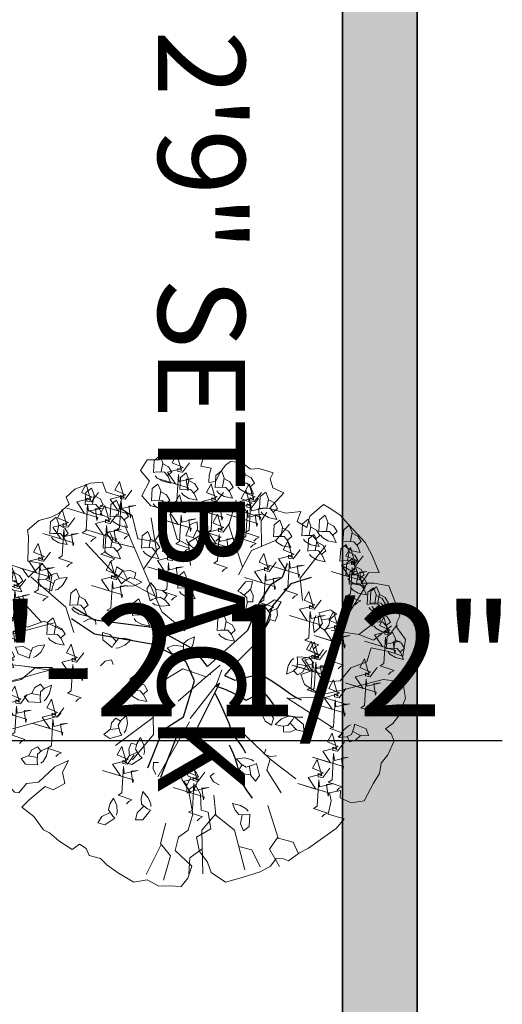
# Model space of a CAD drawing. Units: inches. Extents: x 2337 to 3570, y 1258 to 1938.
# Tile 12 of 30: x 2874 to 2913, y 1598 to 1677. Entities that reach past the tile are written whole.
import ezdxf

# ---------------------------------------------------------------- set-up
doc = ezdxf.new("R2010")
doc.units = ezdxf.units.IN
for name, color, linetype, lineweight in [('A-ANNO-DIMS', 2, 'Continuous', 18), ('A-ANNO-TEXT', 7, 'Continuous', 18), ('ARBOL', 74, 'Continuous', 13), ('C-PROP', 7, 'Continuous', 35)]:
    doc.layers.add(name, color=color, linetype=linetype, lineweight=lineweight)
doc.layers.add('C-PROP-PATT', color=251, linetype='Continuous', lineweight=13, true_color=0x636466)
doc.layers.add('TALLO', color=36, linetype='Continuous')
doc.styles.get("Standard").update_dxf_attribs({"font": 'arial.ttf'})
doc.dimstyles.new('ISO-25', dxfattribs={"dimtxt": 9, "dimasz": 2.5, "dimexe": 1.25, "dimexo": 0.625, "dimtad": 1, "dimdec": 1, "dimlunit": 3, "dimtxsty": 'Standard', "dimcen": 2.5, "dimadec": 0, "dimazin": 0, "dimtfac": 1, "dimtdec": 1, "dimtmove": 0, "dimatfit": 3, "dimfxl": 1, "dimarcsym": 0})

# ---------------------------------------------------------------- blocks, each defined once
blk = doc.blocks.new('fresno')
at = {"layer": 'ARBOL'}
for p, q in [((2.96, 0.991), (3.575, 1.984)), ((-3.638, 1.194), (-4.164, 1.76)), ((-1.151, -0.932), (-1.99, -1.556)), ((-0.974, -3.757), (-1.31, -4.423))]:
    blk.add_line(p, q, dxfattribs=at)
blk.add_lwpolyline([(0.823, 4.745), (0.566, 4.764), (0.459, 4.687), (0.336, 4.518), (0.233, 4.322), (0.087, 4.298), (0.091, 4.464), (0.14, 4.621), (-0.09, 4.659), (-0.033, 4.863), (-0.264, 4.901), (-0.483, 4.866), (-0.686, 4.924), (-1.021, 4.801), (-1.288, 4.8), (-1.431, 4.563), (-1.234, 4.327), (-1.406, 4), (-1.205, 3.778), (-0.909, 3.705), (-0.931, 3.283), (-1.122, 2.983), (-1.491, 3.043), (-1.619, 3.562), (-1.9, 3.727), (-1.851, 3.982), (-2.197, 4.084), (-2.278, 4.31), (-2.543, 4.283), (-2.896, 4.152), (-3.091, 3.971), (-3.022, 3.817), (-3.244, 3.617), (-3.424, 3.528), (-3.697, 3.455), (-3.946, 3.236), (-3.922, 3.09), (-3.94, 2.548), (-3.617, 2.495), (-3.927, 2.19), (-4.062, 2.379), (-4.443, 2.512), (-4.546, 2.316), (-4.73, 2.062), (-4.767, 1.832), (-4.671, 1.698), (-4.486, 1.667), (-4.693, 1.559), (-4.854, 1.444), (-4.934, 1.102), (-5.037, 0.905), (-5.175, 0.644), (-5.166, 0.406), (-5.024, 0.264), (-4.781, 0.153), (-4.363, 0.249), (-4.014, 0.215), (-3.783, 0.177), (-3.46, 0.124), (-3.733, 0.051), (-4.132, -0.073), (-4.404, -0.146), (-4.639, 0.011), (-4.977, -0.028), (-5.172, -0.209), (-5.113, -0.574), (-4.921, -0.843), (-4.951, -1.027), (-5.012, -1.112), (-4.95, -1.311), (-4.83, -1.592), (-4.676, -1.807), (-4.518, -1.856), (-4.529, -2.068), (-4.417, -2.394), (-4.236, -2.59), (-4.143, -2.605), (-3.967, -2.397), (-3.703, -2.37), (-3.339, -2.027), (-3.032, -1.889), (-3.169, -2.15), (-3.115, -2.396), (-3.376, -2.542), (-3.552, -2.466), (-3.909, -2.762), (-4.077, -2.924), (-3.804, -3.135), (-3.592, -3.43), (-3.461, -3.499), (-3.253, -3.676), (-2.953, -3.867), (-2.792, -3.752), (-2.642, -3.848), (-2.572, -4.001), (-2.323, -4.066), (-2.18, -4.208), (-1.926, -4.392), (-1.58, -4.591), (-1.288, -4.545), (-1.027, -4.683), (-0.788, -4.675), (-0.531, -4.693), (-0.382, -4.505), (-0.29, -4.236), (-0.66, -3.891), (-0.588, -3.595), (-0.374, -3.441), (-0.267, -3.079), (-0.368, -2.541), (-0.208, -2.426), (-0.099, -2.633), (-0.087, -2.991), (0.071, -3.04), (0.129, -3.405), (-0.185, -3.59), (-0.119, -3.909), (0.055, -4.151), (0.136, -4.377), (0.456, -4.596), (0.828, -4.491), (1.227, -4.368), (1.461, -4.241), (1.583, -4.071), (1.748, -4.075), (1.86, -4.117), (2.101, -3.944), (2.308, -3.836), (2.925, -3.393), (3.101, -3.185), (2.74, -3.078), (2.812, -2.782), (2.769, -2.61), (3.015, -2.555), (3.012, -2.721), (3.254, -2.832), (3.546, -2.785), (3.752, -2.393), (3.882, -2.177), (3.92, -1.947), (4.069, -1.758), (4.214, -1.451), (4.144, -1.297), (4.021, -1.182), (4.182, -1.067), (4.304, -0.897), (4.464, -0.497), (4.429, -0.279), (4.406, -0.133), (3.964, -0.083), (3.074, -0.315), (2.582, -0.424), (2.217, -0.197), (2.136, 0.029), (2.462, 0.141), (2.628, -0.147), (3.012, -0.116), (3.249, 0.177), (3.602, 0.308), (3.701, 0.623), (4.089, 0.535), (4.404, 0.436), (4.464, 0.805), (4.272, 1.074), (4.267, 1.193), (4.336, 1.324), (4.243, 1.623), (4.092, 2.003), (3.769, 2.057), (3.485, 2.056), (3.642, 2.291), (3.88, 2.299), (3.71, 2.706), (3.563, 2.967), (3.201, 3.358), (3.001, 3.581), (2.766, 3.738), (2.635, 3.807), (2.332, 3.549), (2.268, 3.299), (2.052, 3.429), (2.136, 3.652), (1.798, 3.613), (1.437, 3.72), (1.755, 4.071), (1.513, 4.182), (1.451, 4.381), (1.519, 4.512), (1.204, 4.611), (1.012, 4.596)], close=True, dxfattribs=at)
for points in [[(-1.104, 4.45), (-1.063, 4.399), (-0.939, 4.325), (-0.757, 4.285), (-0.82, 4.431), (-0.903, 4.527), (-1.075, 4.533), (-1.143, 4.521), (-1.126, 4.792), (-1.002, 4.891), (-0.939, 4.738), (-0.975, 4.535)], [(-0.346, 4.735), (-0.501, 4.528), (-0.605, 4.545), (-0.605, 4.614), (-0.519, 4.563), (-0.622, 4.925), (-0.726, 4.735), (-0.484, 4.632), (-0.622, 4.58), (-0.829, 4.528), (-0.657, 4.27), (-1.053, 4.39), (-0.363, 4.183), (-0.381, 4.114), (-0.415, 4.373), (-0.26, 4.39), (-0.57, 4.321), (-0.588, 4.476), (-0.622, 3.89), (-0.708, 3.839), (-0.398, 3.735), (-0.467, 3.701), (-0.519, 3.649)], [(-0.935, 4.717), (-0.809, 4.65), (-0.736, 4.529), (-0.824, 4.459)], [(0.734, 4.203), (0.775, 4.152), (0.9, 4.078), (1.082, 4.038), (1.018, 4.185), (0.936, 4.281), (0.763, 4.287), (0.696, 4.274), (0.712, 4.546), (0.837, 4.645), (0.899, 4.491), (0.863, 4.289)], [(-0.521, 4.069), (-0.48, 4.018), (-0.356, 3.944), (-0.174, 3.904), (-0.237, 4.051), (-0.32, 4.146), (-0.492, 4.152), (-0.56, 4.14), (-0.543, 4.411), (-0.419, 4.511), (-0.356, 4.357), (-0.392, 4.154)], [(0.263, 4.114), (0.304, 4.063), (0.429, 3.989), (0.611, 3.948), (0.547, 4.095), (0.465, 4.191), (0.293, 4.197), (0.225, 4.185), (0.242, 4.456), (0.366, 4.555), (0.428, 4.402), (0.393, 4.199)], [(0.904, 4.471), (1.029, 4.404), (1.102, 4.282), (1.015, 4.212)], [(-2.368, 4.073), (-2.523, 3.866), (-2.627, 3.883), (-2.627, 3.952), (-2.541, 3.9), (-2.644, 4.262), (-2.748, 4.073), (-2.506, 3.969), (-2.644, 3.918), (-2.851, 3.866), (-2.679, 3.607), (-3.075, 3.728), (-2.385, 3.521), (-2.403, 3.452), (-2.437, 3.711), (-2.282, 3.728), (-2.592, 3.659), (-2.61, 3.814), (-2.644, 3.228), (-2.73, 3.176), (-2.42, 3.073), (-2.489, 3.038), (-2.541, 2.987)], [(-2.629, 3.733), (-2.588, 3.682), (-2.463, 3.608), (-2.281, 3.568), (-2.345, 3.715), (-2.427, 3.81), (-2.6, 3.816), (-2.667, 3.804), (-2.651, 4.075), (-2.526, 4.175), (-2.464, 4.021), (-2.5, 3.818)], [(-1.623, 4.132), (-1.778, 3.925), (-1.882, 3.942), (-1.882, 4.011), (-1.795, 3.959), (-1.899, 4.321), (-2.002, 4.132), (-1.761, 4.028), (-1.899, 3.977), (-2.106, 3.925), (-1.933, 3.666), (-2.33, 3.787), (-1.64, 3.58), (-1.657, 3.511), (-1.692, 3.77), (-1.537, 3.787), (-1.847, 3.718), (-1.864, 3.873), (-1.899, 3.287), (-1.985, 3.235), (-1.675, 3.132), (-1.744, 3.097), (-1.795, 3.046)], [(-1.149, 3.822), (-1.108, 3.771), (-0.983, 3.697), (-0.802, 3.657), (-0.865, 3.804), (-0.948, 3.9), (-1.12, 3.906), (-1.188, 3.893), (-1.171, 4.165), (-1.047, 4.264), (-0.984, 4.111), (-1.02, 3.908)], [(-0.352, 4.337), (-0.226, 4.269), (-0.153, 4.148), (-0.241, 4.078)], [(0.413, 4.08), (0.258, 3.873), (0.154, 3.89), (0.154, 3.959), (0.241, 3.908), (0.137, 4.27), (0.034, 4.08), (0.275, 3.977), (0.137, 3.925), (-0.07, 3.873), (0.103, 3.614), (-0.294, 3.735), (0.396, 3.528), (0.379, 3.459), (0.344, 3.718), (0.499, 3.735), (0.189, 3.666), (0.172, 3.821), (0.137, 3.235), (0.051, 3.183), (0.361, 3.08), (0.292, 3.046), (0.241, 2.994)], [(0.433, 4.381), (0.558, 4.314), (0.631, 4.193), (0.544, 4.122)], [(1.259, 4.08), (1.103, 3.873), (1, 3.89), (1, 3.959), (1.086, 3.908), (0.982, 4.27), (0.879, 4.08), (1.12, 3.977), (0.982, 3.925), (0.775, 3.873), (0.948, 3.614), (0.551, 3.735), (1.241, 3.528), (1.224, 3.459), (1.189, 3.718), (1.345, 3.735), (1.034, 3.666), (1.017, 3.821), (0.982, 3.235), (0.896, 3.183), (1.207, 3.08), (1.138, 3.046), (1.086, 2.994)], [(-2.459, 4), (-2.334, 3.933), (-2.261, 3.812), (-2.348, 3.742)], [(-0.287, 3.833), (-0.442, 3.626), (-0.546, 3.643), (-0.546, 3.712), (-0.46, 3.661), (-0.563, 4.023), (-0.667, 3.833), (-0.425, 3.73), (-0.563, 3.678), (-0.77, 3.626), (-0.598, 3.367), (-0.995, 3.488), (-0.304, 3.281), (-0.322, 3.212), (-0.356, 3.471), (-0.201, 3.488), (-0.511, 3.419), (-0.529, 3.574), (-0.563, 2.988), (-0.649, 2.936), (-0.339, 2.833), (-0.408, 2.799), (-0.46, 2.747)], [(-0.98, 4.09), (-0.854, 4.023), (-0.781, 3.901), (-0.869, 3.831)], [(1.189, 3.942), (1.034, 3.735), (0.931, 3.752), (0.931, 3.821), (1.017, 3.77), (0.913, 4.132), (0.81, 3.942), (1.051, 3.839), (0.913, 3.787), (0.706, 3.735), (0.879, 3.477), (0.482, 3.597), (1.172, 3.39), (1.155, 3.321), (1.12, 3.58), (1.276, 3.597), (0.965, 3.528), (0.948, 3.683), (0.913, 3.097), (0.827, 3.046), (1.138, 2.942), (1.069, 2.908), (1.017, 2.856)], [(1.25, 3.643), (1.291, 3.592), (1.416, 3.518), (1.597, 3.478), (1.534, 3.625), (1.451, 3.721), (1.279, 3.727), (1.211, 3.714), (1.228, 3.985), (1.352, 4.085), (1.415, 3.931), (1.379, 3.729)], [(-1.951, 3.597), (-2.106, 3.39), (-2.209, 3.408), (-2.209, 3.477), (-2.123, 3.425), (-2.227, 3.787), (-2.33, 3.597), (-2.089, 3.494), (-2.227, 3.442), (-2.434, 3.39), (-2.261, 3.132), (-2.658, 3.252), (-1.968, 3.046), (-1.985, 2.977), (-2.02, 3.235), (-1.864, 3.252), (-2.175, 3.183), (-2.192, 3.339), (-2.227, 2.752), (-2.313, 2.701), (-2.002, 2.597), (-2.071, 2.563), (-2.123, 2.511)], [(-2.068, 3.464), (-2.027, 3.413), (-1.903, 3.339), (-1.721, 3.299), (-1.784, 3.446), (-1.867, 3.542), (-2.039, 3.547), (-2.107, 3.535), (-2.09, 3.806), (-1.966, 3.906), (-1.903, 3.752), (-1.939, 3.55)], [(-1.899, 3.732), (-1.773, 3.664), (-1.7, 3.543), (-1.788, 3.473)], [(0.837, 2.414), (0.533, 3.352), (0.697, 3.906)], [(1.419, 3.911), (1.545, 3.844), (1.618, 3.722), (1.53, 3.652)], [(-2.898, 3.511), (-3.053, 3.304), (-3.157, 3.321), (-3.157, 3.39), (-3.071, 3.339), (-3.174, 3.701), (-3.278, 3.511), (-3.036, 3.408), (-3.174, 3.356), (-3.381, 3.304), (-3.209, 3.046), (-3.605, 3.166), (-2.915, 2.959), (-2.932, 2.89), (-2.967, 3.149), (-2.812, 3.166), (-3.122, 3.097), (-3.14, 3.253), (-3.174, 2.666), (-3.26, 2.615), (-2.95, 2.511), (-3.019, 2.477), (-3.071, 2.425)], [(-3.413, 3.083), (-3.373, 3.032), (-3.248, 2.958), (-3.066, 2.918), (-3.129, 3.065), (-3.212, 3.161), (-3.384, 3.167), (-3.452, 3.154), (-3.435, 3.425), (-3.311, 3.525), (-3.248, 3.371), (-3.284, 3.169)], [(-1.367, 2.367), (-1.081, 2.78), (-1.193, 3.514)], [(-0.358, 2.895), (-0.615, 3.037), (-0.783, 3.596)], [(-0.063, 3.671), (-0.069, 3.151), (-0.364, 2.965), (-0.319, 2.449)], [(0.558, 3.402), (0.403, 3.195), (0.299, 3.212), (0.299, 3.281), (0.386, 3.23), (0.282, 3.592), (0.179, 3.402), (0.42, 3.299), (0.282, 3.247), (0.075, 3.195), (0.248, 2.936), (-0.149, 3.057), (0.541, 2.85), (0.524, 2.781), (0.489, 3.04), (0.644, 3.057), (0.334, 2.988), (0.317, 3.143), (0.282, 2.557), (0.196, 2.505), (0.506, 2.402), (0.437, 2.368), (0.386, 2.316)], [(1.259, 2.882), (1.254, 3.446), (1.381, 3.636)], [(2.573, 3.128), (2.613, 3.077), (2.738, 3.003), (2.92, 2.963), (2.857, 3.11), (2.774, 3.205), (2.602, 3.211), (2.534, 3.199), (2.551, 3.47), (2.675, 3.57), (2.738, 3.416), (2.702, 3.214)], [(-3.244, 3.351), (-3.118, 3.284), (-3.045, 3.162), (-3.133, 3.092)], [(-0.448, 1), (-0.961, 1.419), (-1.784, 3.341)], [(-0.923, 3.449), (-0.951, 3.425), (-0.93, 3.313)], [(-0.41, 3.035), (-0.387, 2.974), (-0.291, 2.865), (-0.131, 2.771), (-0.146, 2.93), (-0.195, 3.047), (-0.357, 3.106), (-0.425, 3.115), (-0.325, 3.368), (-0.176, 3.424), (-0.164, 3.258), (-0.261, 3.077)], [(0.746, 2.242), (1.034, 2.786), (1.584, 3.019), (1.879, 3.374)], [(1.564, 3.016), (1.605, 2.965), (1.729, 2.891), (1.911, 2.851), (1.848, 2.998), (1.765, 3.094), (1.593, 3.099), (1.525, 3.087), (1.542, 3.358), (1.666, 3.458), (1.729, 3.304), (1.693, 3.102)], [(2.191, 3.038), (2.232, 2.987), (2.357, 2.913), (2.539, 2.873), (2.475, 3.02), (2.393, 3.116), (2.221, 3.122), (2.153, 3.109), (2.17, 3.381), (2.294, 3.48), (2.356, 3.326), (2.321, 3.124)], [(2.361, 3.306), (2.486, 3.239), (2.559, 3.117), (2.472, 3.047)], [(2.742, 3.396), (2.868, 3.328), (2.941, 3.207), (2.853, 3.137)], [(3.111, 2.904), (3.152, 2.853), (3.276, 2.779), (3.458, 2.739), (3.395, 2.886), (3.312, 2.981), (3.14, 2.987), (3.072, 2.975), (3.089, 3.246), (3.213, 3.346), (3.276, 3.192), (3.24, 2.99)], [(-2.225, 2.77), (-2.184, 2.718), (-2.06, 2.645), (-1.878, 2.604), (-1.941, 2.751), (-2.024, 2.847), (-2.196, 2.853), (-2.264, 2.84), (-2.247, 3.112), (-2.123, 3.211), (-2.06, 3.058), (-2.096, 2.855)], [(-1.575, 2.854), (-2.052, 2.969), (-2.2, 3.178)], [(-1.373, 2.77), (-1.332, 2.718), (-1.208, 2.645), (-1.026, 2.604), (-1.089, 2.751), (-1.172, 2.847), (-1.344, 2.853), (-1.412, 2.84), (-1.395, 3.112), (-1.271, 3.211), (-1.208, 3.058), (-1.244, 2.855)], [(-0.166, 3.238), (-0.068, 3.135), (-0.036, 2.997), (-0.141, 2.957)], [(1.733, 3.284), (1.859, 3.216), (1.932, 3.095), (1.844, 3.025)], [(2.326, 2.702), (2.367, 2.651), (2.492, 2.577), (2.673, 2.537), (2.61, 2.684), (2.527, 2.78), (2.355, 2.786), (2.287, 2.773), (2.304, 3.045), (2.428, 3.144), (2.491, 2.99), (2.455, 2.788)], [(3.28, 3.172), (3.406, 3.104), (3.479, 2.983), (3.391, 2.913)], [(-3.434, 2.752), (-3.59, 2.546), (-3.693, 2.563), (-3.693, 2.632), (-3.607, 2.58), (-3.71, 2.942), (-3.814, 2.752), (-3.572, 2.649), (-3.71, 2.597), (-3.917, 2.546), (-3.745, 2.287), (-4.142, 2.408), (-3.452, 2.201), (-3.469, 2.132), (-3.503, 2.39), (-3.348, 2.408), (-3.659, 2.339), (-3.676, 2.494), (-3.71, 1.908), (-3.797, 1.856), (-3.486, 1.753), (-3.555, 1.718), (-3.607, 1.666)], [(-1.112, 1.773), (-2.014, 2.265), (-2.654, 2.957)], [(-2.056, 3.037), (-1.93, 2.97), (-1.857, 2.849), (-1.945, 2.778)], [(-0.57, 2.77), (-0.726, 2.563), (-0.829, 2.58), (-0.829, 2.649), (-0.743, 2.597), (-0.846, 2.959), (-0.95, 2.77), (-0.708, 2.666), (-0.846, 2.615), (-1.053, 2.563), (-0.881, 2.304), (-1.278, 2.425), (-0.588, 2.218), (-0.605, 2.149), (-0.639, 2.408), (-0.484, 2.425), (-0.795, 2.356), (-0.812, 2.511), (-0.846, 1.925), (-0.933, 1.873), (-0.622, 1.77), (-0.691, 1.735), (-0.743, 1.684)], [(-1.204, 3.037), (-1.078, 2.97), (-1.005, 2.849), (-1.093, 2.778)], [(2.121, 2.804), (1.966, 2.597), (1.862, 2.615), (1.862, 2.683), (1.949, 2.632), (1.845, 2.994), (1.742, 2.804), (1.983, 2.701), (1.845, 2.649), (1.638, 2.597), (1.811, 2.339), (1.414, 2.459), (2.104, 2.252), (2.087, 2.184), (2.052, 2.442), (2.207, 2.459), (1.897, 2.39), (1.88, 2.546), (1.845, 1.959), (1.759, 1.908), (2.069, 1.804), (2, 1.77), (1.949, 1.718)], [(2.171, 1.674), (2.121, 2.172), (2.689, 2.898)], [(2.495, 2.97), (2.621, 2.903), (2.694, 2.781), (2.606, 2.711)], [(3.519, 2.666), (3.363, 2.459), (3.26, 2.477), (3.26, 2.546), (3.346, 2.494), (3.243, 2.856), (3.139, 2.666), (3.381, 2.563), (3.243, 2.511), (3.036, 2.459), (3.208, 2.201), (2.811, 2.321), (3.501, 2.115), (3.484, 2.046), (3.45, 2.304), (3.605, 2.321), (3.294, 2.252), (3.277, 2.408), (3.243, 1.821), (3.156, 1.77), (3.467, 1.666), (3.398, 1.632), (3.346, 1.58)], [(3.043, 2.478), (3.084, 2.427), (3.209, 2.353), (3.391, 2.313), (3.327, 2.46), (3.245, 2.556), (3.073, 2.562), (3.005, 2.549), (3.022, 2.82), (3.146, 2.92), (3.208, 2.766), (3.173, 2.564)], [(1.586, 2.528), (1.431, 2.321), (1.327, 2.339), (1.327, 2.408), (1.414, 2.356), (1.31, 2.718), (1.207, 2.528), (1.448, 2.425), (1.31, 2.373), (1.103, 2.321), (1.276, 2.063), (0.879, 2.184), (1.569, 1.977), (1.552, 1.908), (1.517, 2.166), (1.673, 2.184), (1.362, 2.115), (1.345, 2.27), (1.31, 1.684), (1.224, 1.632), (1.535, 1.528), (1.466, 1.494), (1.414, 1.442)], [(3.213, 2.746), (3.338, 2.679), (3.411, 2.557), (3.324, 2.487)], [(-4.422, 2.03), (-4.381, 1.979), (-4.257, 1.905), (-4.075, 1.865), (-4.138, 2.012), (-4.221, 2.108), (-4.393, 2.114), (-4.461, 2.101), (-4.444, 2.372), (-4.32, 2.472), (-4.257, 2.318), (-4.293, 2.116)], [(-3.468, 1.85), (-3.409, 2.222), (-3.628, 2.505)], [(-1.817, 2.351), (-1.972, 2.144), (-2.075, 2.162), (-2.075, 2.231), (-1.989, 2.179), (-2.093, 2.541), (-2.196, 2.351), (-1.955, 2.248), (-2.093, 2.196), (-2.3, 2.144), (-2.127, 1.886), (-2.524, 2.006), (-1.834, 1.8), (-1.851, 1.731), (-1.886, 1.989), (-1.73, 2.006), (-2.041, 1.937), (-2.058, 2.093), (-2.093, 1.506), (-2.179, 1.455), (-1.868, 1.351), (-1.937, 1.317), (-1.989, 1.265)], [(-1.786, 2.007), (-1.722, 1.99), (-1.578, 2.003), (-1.407, 2.078), (-1.545, 2.159), (-1.668, 2.188), (-1.811, 2.092), (-1.859, 2.042), (-2.004, 2.271), (-1.962, 2.425), (-1.821, 2.337), (-1.731, 2.152)], [(3.178, 2.165), (3.219, 2.113), (3.344, 2.04), (3.525, 1.999), (3.462, 2.146), (3.379, 2.242), (3.207, 2.248), (3.139, 2.236), (3.156, 2.507), (3.28, 2.606), (3.343, 2.453), (3.307, 2.25)], [(3.347, 2.432), (3.473, 2.365), (3.546, 2.244), (3.458, 2.173)], [(-3.986, 2.149), (-4.142, 1.942), (-4.245, 1.959), (-4.245, 2.028), (-4.159, 1.977), (-4.262, 2.339), (-4.366, 2.149), (-4.124, 2.046), (-4.262, 1.994), (-4.47, 1.942), (-4.297, 1.684), (-4.694, 1.804), (-4.004, 1.597), (-4.021, 1.528), (-4.055, 1.787), (-3.9, 1.804), (-4.211, 1.735), (-4.228, 1.89), (-4.262, 1.304), (-4.349, 1.253), (-4.038, 1.149), (-4.107, 1.115), (-4.159, 1.063)], [(-4.253, 2.298), (-4.127, 2.231), (-4.054, 2.109), (-4.142, 2.039)], [(-2.916, 0.958), (-3.096, 1.528), (-3.871, 2.197)], [(-3.533, 2.149), (-3.43, 2.247), (-3.292, 2.279), (-3.252, 2.174)], [(-1.806, 2.323), (-1.665, 2.343), (-1.534, 2.287), (-1.564, 2.179)], [(-0.566, 1.873), (-0.525, 1.822), (-0.4, 1.748), (-0.219, 1.708), (-0.282, 1.855), (-0.365, 1.951), (-0.537, 1.957), (-0.605, 1.944), (-0.588, 2.216), (-0.464, 2.315), (-0.401, 2.162), (-0.437, 1.959)], [(3.245, 1.963), (3.286, 1.912), (3.411, 1.838), (3.593, 1.798), (3.529, 1.945), (3.447, 2.041), (3.274, 2.046), (3.206, 2.034), (3.223, 2.305), (3.347, 2.405), (3.41, 2.251), (3.374, 2.049)], [(3.415, 2.231), (3.54, 2.163), (3.613, 2.042), (3.525, 1.972)], [(-3.331, 1.905), (-3.269, 1.928), (-3.161, 2.024), (-3.066, 2.184), (-3.226, 2.169), (-3.342, 2.121), (-3.401, 1.958), (-3.41, 1.89), (-3.663, 1.99), (-3.719, 2.139), (-3.554, 2.151), (-3.372, 2.054)], [(-1.164, 1.612), (-1.109, 1.576), (-0.967, 1.544), (-0.782, 1.562), (-0.888, 1.682), (-0.996, 1.748), (-1.162, 1.7), (-1.222, 1.667), (-1.29, 1.93), (-1.203, 2.063), (-1.096, 1.937), (-1.067, 1.733)], [(-0.397, 2.141), (-0.271, 2.074), (-0.198, 1.952), (-0.286, 1.882)], [(0.72, 1.798), (0.723, 1.733), (0.781, 1.6), (0.904, 1.46), (0.939, 1.616), (0.929, 1.742), (0.793, 1.848), (0.73, 1.878), (0.904, 2.088), (1.062, 2.095), (1.023, 1.934), (0.875, 1.791)], [(3.716, 1.537), (3.757, 1.486), (3.882, 1.412), (4.063, 1.372), (4, 1.519), (3.917, 1.615), (3.745, 1.621), (3.677, 1.608), (3.694, 1.88), (3.818, 1.979), (3.881, 1.825), (3.845, 1.623)], [(-2.965, 1.493), (-2.924, 1.441), (-2.799, 1.368), (-2.618, 1.327), (-2.681, 1.474), (-2.764, 1.57), (-2.936, 1.576), (-3.004, 1.564), (-2.987, 1.835), (-2.863, 1.934), (-2.8, 1.781), (-2.836, 1.578)], [(-2.796, 1.76), (-2.67, 1.693), (-2.597, 1.572), (-2.685, 1.501)], [(-1.085, 1.919), (-0.945, 1.893), (-0.838, 1.801), (-0.9, 1.707)], [(1.014, 1.915), (1.077, 1.787), (1.064, 1.646), (0.952, 1.64)], [(2.587, 1.684), (2.432, 1.477), (2.328, 1.494), (2.328, 1.563), (2.414, 1.511), (2.311, 1.873), (2.207, 1.684), (2.449, 1.58), (2.311, 1.528), (2.104, 1.477), (2.276, 1.218), (1.88, 1.339), (2.57, 1.132), (2.552, 1.063), (2.518, 1.321), (2.673, 1.339), (2.363, 1.27), (2.345, 1.425), (2.311, 0.839), (2.225, 0.787), (2.535, 0.684), (2.466, 0.649), (2.414, 0.597)], [(3.649, 1.515), (3.69, 1.464), (3.814, 1.39), (3.996, 1.35), (3.933, 1.497), (3.85, 1.592), (3.678, 1.598), (3.61, 1.586), (3.627, 1.857), (3.751, 1.957), (3.814, 1.803), (3.778, 1.601)], [(3.818, 1.783), (3.944, 1.715), (4.017, 1.594), (3.929, 1.524)], [(3.885, 1.805), (4.011, 1.738), (4.084, 1.616), (3.996, 1.546)], [(-4.193, 1.356), (-4.349, 1.149), (-4.452, 1.166), (-4.452, 1.235), (-4.366, 1.184), (-4.469, 1.546), (-4.573, 1.356), (-4.331, 1.253), (-4.469, 1.201), (-4.677, 1.149), (-4.504, 0.89), (-4.901, 1.011), (-4.211, 0.804), (-4.228, 0.735), (-4.262, 0.994), (-4.107, 1.011), (-4.418, 0.942), (-4.435, 1.097), (-4.469, 0.511), (-4.556, 0.459), (-4.245, 0.356), (-4.314, 0.322), (-4.366, 0.27)], [(-4.759, 1.269), (-4.718, 1.217), (-4.593, 1.144), (-4.411, 1.103), (-4.475, 1.25), (-4.557, 1.346), (-4.729, 1.352), (-4.797, 1.339), (-4.78, 1.611), (-4.656, 1.71), (-4.594, 1.557), (-4.629, 1.354)], [(-4.589, 1.536), (-4.464, 1.469), (-4.391, 1.348), (-4.478, 1.277)], [(-1.575, 1.269), (-1.534, 1.217), (-1.409, 1.144), (-1.228, 1.103), (-1.291, 1.25), (-1.373, 1.346), (-1.546, 1.352), (-1.614, 1.339), (-1.597, 1.611), (-1.473, 1.71), (-1.41, 1.557), (-1.446, 1.354)], [(-1.406, 1.536), (-1.28, 1.469), (-1.207, 1.348), (-1.295, 1.277)], [(1.283, 1.469), (1.266, 1.405), (1.279, 1.261), (1.354, 1.09), (1.435, 1.228), (1.464, 1.351), (1.368, 1.494), (1.318, 1.542), (1.547, 1.687), (1.7, 1.645), (1.613, 1.504), (1.428, 1.414)], [(3.761, 1.112), (3.802, 1.061), (3.926, 0.987), (4.108, 0.947), (4.045, 1.093), (3.962, 1.189), (3.79, 1.195), (3.722, 1.183), (3.739, 1.454), (3.863, 1.553), (3.926, 1.4), (3.89, 1.197)], [(-3.192, 1.017), (-3.578, 1.215), (-3.949, 1.081), (-4.398, 1.339)], [(0.308, 0.933), (0.349, 0.881), (0.474, 0.807), (0.656, 0.767), (0.592, 0.914), (0.51, 1.01), (0.337, 1.016), (0.27, 1.003), (0.286, 1.275), (0.411, 1.374), (0.473, 1.221), (0.437, 1.018)], [(1.599, 1.489), (1.618, 1.348), (1.563, 1.217), (1.455, 1.247)], [(2.479, 1.34), (2.443, 1.285), (2.411, 1.143), (2.429, 0.958), (2.549, 1.064), (2.615, 1.172), (2.567, 1.338), (2.534, 1.398), (2.797, 1.466), (2.93, 1.379), (2.804, 1.272), (2.6, 1.243)], [(3.139, 1.235), (2.984, 1.028), (2.88, 1.046), (2.88, 1.115), (2.967, 1.063), (2.863, 1.425), (2.759, 1.235), (3.001, 1.132), (2.863, 1.08), (2.656, 1.028), (2.828, 0.77), (2.432, 0.891), (3.122, 0.684), (3.105, 0.615), (3.07, 0.873), (3.225, 0.891), (2.915, 0.822), (2.897, 0.977), (2.863, 0.391), (2.777, 0.339), (3.087, 0.235), (3.018, 0.201), (2.967, 0.149)], [(4.01, 1.36), (3.422, 0.918)], [(3.93, 1.379), (4.056, 1.312), (4.129, 1.191), (4.041, 1.121)], [(-3.354, 1.176), (-4.529, 0.864)], [(-3.481, 0.843), (-3.44, 0.792), (-3.315, 0.718), (-3.133, 0.678), (-3.197, 0.825), (-3.279, 0.92), (-3.451, 0.926), (-3.519, 0.914), (-3.502, 1.185), (-3.378, 1.285), (-3.316, 1.131), (-3.351, 0.928)], [(-3.311, 1.111), (-3.186, 1.043), (-3.113, 0.922), (-3.2, 0.852)], [(-2.703, 1.201), (-2.575, 1.263), (-2.433, 1.251), (-2.428, 1.139)], [(0.478, 1.2), (0.603, 1.133), (0.676, 1.011), (0.589, 0.941)], [(2.786, 1.261), (2.76, 1.121), (2.668, 1.014), (2.574, 1.076)], [(2.808, 1.015), (3.422, 0.918), (3.422, 0.918), (3.748, 0.794), (4.154, 1.111)], [(4.26, 1.115), (4.105, 0.908), (4.002, 0.925), (4.002, 0.994), (4.088, 0.942), (3.984, 1.304), (3.881, 1.115), (4.122, 1.011), (3.984, 0.959), (3.777, 0.908), (3.95, 0.649), (3.553, 0.77), (4.243, 0.563), (4.226, 0.494), (4.191, 0.753), (4.347, 0.77), (4.036, 0.701), (4.019, 0.856), (3.984, 0.27), (3.898, 0.218), (4.209, 0.115), (4.14, 0.08), (4.088, 0.029)], [(-5.028, 0.44), (-4.987, 0.388), (-4.862, 0.315), (-4.68, 0.274), (-4.744, 0.421), (-4.826, 0.517), (-4.998, 0.523), (-5.066, 0.511), (-5.049, 0.782), (-4.925, 0.881), (-4.863, 0.728), (-4.898, 0.525)], [(-1.981, 0.615), (-1.915, 0.618), (-1.782, 0.676), (-1.643, 0.799), (-1.799, 0.834), (-1.925, 0.824), (-2.031, 0.688), (-2.061, 0.626), (-2.27, 0.799), (-2.278, 0.958), (-2.117, 0.918), (-1.974, 0.77)], [(4.075, 0.529), (4.116, 0.478), (4.24, 0.404), (4.422, 0.364), (4.359, 0.511), (4.276, 0.607), (4.104, 0.613), (4.036, 0.6), (4.053, 0.871), (4.177, 0.971), (4.24, 0.817), (4.204, 0.615)], [(-4.858, 0.707), (-4.733, 0.64), (-4.66, 0.519), (-4.747, 0.448)], [(-4.602, 0.35), (-4.561, 0.299), (-4.436, 0.225), (-4.254, 0.185), (-4.318, 0.332), (-4.4, 0.428), (-4.572, 0.433), (-4.64, 0.421), (-4.623, 0.692), (-4.499, 0.792), (-4.437, 0.638), (-4.472, 0.436)], [(-3.824, 0.404), (-3.763, 0.427), (-3.654, 0.523), (-3.559, 0.683), (-3.719, 0.668), (-3.835, 0.62), (-3.894, 0.457), (-3.903, 0.389), (-4.156, 0.489), (-4.212, 0.638), (-4.047, 0.65), (-3.865, 0.553)], [(-2.698, 0.509), (-2.854, 0.302), (-2.957, 0.319), (-2.957, 0.388), (-2.871, 0.336), (-2.974, 0.698), (-3.078, 0.509), (-2.836, 0.405), (-2.974, 0.353), (-3.182, 0.302), (-3.009, 0.043), (-3.406, 0.164), (-2.716, -0.043), (-2.733, -0.112), (-2.767, 0.147), (-2.612, 0.164), (-2.923, 0.095), (-2.94, 0.25), (-2.974, -0.336), (-3.061, -0.388), (-2.75, -0.491), (-2.819, -0.526), (-2.871, -0.577)], [(-0.397, 0.517), (-0.346, 0.557), (-0.272, 0.682), (-0.232, 0.864), (-0.379, 0.801), (-0.474, 0.718), (-0.48, 0.546), (-0.468, 0.478), (-0.739, 0.495), (-0.838, 0.619), (-0.685, 0.682), (-0.482, 0.646)], [(2.639, 0.58), (2.483, 0.373), (2.38, 0.391), (2.38, 0.46), (2.466, 0.408), (2.363, 0.77), (2.259, 0.58), (2.501, 0.477), (2.363, 0.425), (2.156, 0.373), (2.328, 0.115), (1.931, 0.235), (2.621, 0.029), (2.604, -0.04), (2.57, 0.218), (2.725, 0.235), (2.414, 0.166), (2.397, 0.322), (2.363, -0.265), (2.276, -0.316), (2.587, -0.42), (2.518, -0.454), (2.466, -0.506)], [(2.708, 0.563), (2.552, 0.356), (2.449, 0.373), (2.449, 0.442), (2.535, 0.391), (2.432, 0.753), (2.328, 0.563), (2.57, 0.46), (2.432, 0.408), (2.225, 0.356), (2.397, 0.097), (2, 0.218), (2.69, 0.011), (2.673, -0.058), (2.639, 0.201), (2.794, 0.218), (2.483, 0.149), (2.466, 0.304), (2.432, -0.282), (2.345, -0.334), (2.656, -0.437), (2.587, -0.471), (2.535, -0.523)], [(4.244, 0.797), (4.37, 0.73), (4.443, 0.608), (4.355, 0.538)], [(-4.432, 0.618), (-4.307, 0.55), (-4.234, 0.429), (-4.321, 0.359)], [(-3.394, 0.18), (-3.77, 0.182), (-4.532, 0.27)], [(-2.322, 0.222), (-2.219, 0.321), (-2.081, 0.353), (-2.042, 0.248)], [(-0.596, -0.564), (0.03, -0.026), (0.339, 0.235)], [(1.978, 0.384), (1.927, 0.343), (1.853, 0.218), (1.813, 0.036), (1.96, 0.1), (2.056, 0.182), (2.061, 0.355), (2.049, 0.422), (2.32, 0.406), (2.42, 0.281), (2.266, 0.219), (2.064, 0.254)], [(3.829, 0.184), (3.674, -0.023), (3.57, -0.006), (3.57, 0.063), (3.657, 0.011), (3.553, 0.373), (3.45, 0.184), (3.691, 0.08), (3.553, 0.029), (3.346, -0.023), (3.519, -0.282), (3.122, -0.161), (3.812, -0.368), (3.795, -0.437), (3.76, -0.178), (3.915, -0.161), (3.605, -0.23), (3.588, -0.075), (3.553, -0.661), (3.467, -0.713), (3.777, -0.816), (3.708, -0.851), (3.657, -0.902)], [(-3.77, 0.182), (-4.09, -0.088), (-4.494, -0.18)], [(-1.642, -0.412), (-1.601, -0.463), (-1.477, -0.537), (-1.295, -0.577), (-1.358, -0.43), (-1.441, -0.334), (-1.613, -0.328), (-1.681, -0.341), (-1.664, -0.069), (-1.54, 0.03), (-1.477, -0.124), (-1.513, -0.326)], [(0.03, -0.026), (-0.491, 0.154), (-0.871, -0.08)], [(0.38, 0.131), (0.248, -0.21), (-0.33, -0.951)], [(2.246, 0.214), (2.178, 0.089), (2.057, 0.016), (1.987, 0.103)], [(-4.871, -0.524), (-4.83, -0.575), (-4.705, -0.649), (-4.523, -0.689), (-4.587, -0.542), (-4.669, -0.446), (-4.841, -0.44), (-4.909, -0.453), (-4.893, -0.181), (-4.768, -0.082), (-4.706, -0.236), (-4.741, -0.438)], [(-3.58, -0.559), (-3.529, -0.518), (-3.455, -0.393), (-3.415, -0.211), (-3.562, -0.275), (-3.658, -0.357), (-3.664, -0.53), (-3.651, -0.597), (-3.923, -0.581), (-4.022, -0.456), (-3.868, -0.394), (-3.666, -0.43)], [(-3.848, -0.389), (-3.781, -0.264), (-3.659, -0.191), (-3.589, -0.278)], [(-1.473, -0.144), (-1.347, -0.211), (-1.274, -0.333), (-1.362, -0.403)], [(3.139, -0.282), (2.984, -0.489), (2.88, -0.471), (2.88, -0.402), (2.967, -0.454), (2.863, -0.092), (2.759, -0.282), (3.001, -0.385), (2.863, -0.437), (2.656, -0.489), (2.828, -0.747), (2.432, -0.627), (3.122, -0.834), (3.105, -0.902), (3.07, -0.644), (3.225, -0.627), (2.915, -0.696), (2.897, -0.54), (2.863, -1.127), (2.777, -1.178), (3.087, -1.282), (3.018, -1.316), (2.967, -1.368)], [(-4.701, -0.256), (-4.576, -0.323), (-4.503, -0.445), (-4.59, -0.515)], [(-3.952, -0.42), (-4.107, -0.627), (-4.211, -0.609), (-4.211, -0.54), (-4.124, -0.592), (-4.228, -0.23), (-4.331, -0.42), (-4.09, -0.523), (-4.228, -0.575), (-4.435, -0.627), (-4.262, -0.885), (-4.659, -0.765), (-3.969, -0.971), (-3.986, -1.04), (-4.021, -0.782), (-3.866, -0.765), (-4.176, -0.834), (-4.193, -0.678), (-4.228, -1.265), (-4.314, -1.316), (-4.004, -1.42), (-4.073, -1.454), (-4.124, -1.506)], [(-3.141, -0.713), (-3.296, -0.92), (-3.4, -0.902), (-3.4, -0.834), (-3.314, -0.885), (-3.417, -0.523), (-3.521, -0.713), (-3.279, -0.816), (-3.417, -0.868), (-3.624, -0.92), (-3.452, -1.178), (-3.848, -1.058), (-3.158, -1.265), (-3.175, -1.333), (-3.21, -1.075), (-3.055, -1.058), (-3.365, -1.127), (-3.383, -0.971), (-3.417, -1.558), (-3.503, -1.609), (-3.193, -1.713), (-3.262, -1.747), (-3.314, -1.799)], [(1.822, -0.495), (2.859, -1.165)], [(1.846, -0.51), (2.605, -0.469), (3.129, -0.637)], [(-3.195, -0.824), (-3.267, -0.898), (-4.285, -1.185)], [(-1.047, -0.767), (-1.151, -0.913), (-1.144, -1.307), (-1.61, -1.871)], [(1.304, -0.681), (1.241, -0.664), (1.097, -0.678), (0.926, -0.752), (1.064, -0.833), (1.187, -0.862), (1.33, -0.766), (1.377, -0.716), (1.523, -0.945), (1.481, -1.099), (1.34, -1.011), (1.25, -0.826)], [(-1.794, -1.268), (-1.758, -1.214), (-1.726, -1.072), (-1.744, -0.887), (-1.865, -0.993), (-1.93, -1.101), (-1.883, -1.266), (-1.85, -1.327), (-2.113, -1.395), (-2.246, -1.307), (-2.119, -1.2), (-1.916, -1.172)], [(-2.101, -1.19), (-2.076, -1.05), (-1.983, -0.943), (-1.889, -1.004)], [(-0.346, -1.024), (-1.05, -2.251)], [(1.903, -0.903), (1.837, -0.905), (1.704, -0.963), (1.565, -1.086), (1.721, -1.122), (1.847, -1.111), (1.953, -0.975), (1.983, -0.913), (2.192, -1.086), (2.2, -1.245), (2.039, -1.205), (1.896, -1.057)], [(3.253, -1.094), (3.192, -1.117), (3.083, -1.213), (2.988, -1.374), (3.148, -1.359), (3.264, -1.31), (3.323, -1.148), (3.332, -1.079), (3.585, -1.179), (3.641, -1.328), (3.476, -1.34), (3.294, -1.244)], [(0.748, -1.185), (1.452, -1.855), (2.021, -2.292)], [(2.02, -1.197), (1.891, -1.259), (1.75, -1.247), (1.745, -1.134)], [(3.105, -1.471), (2.949, -1.678), (2.846, -1.661), (2.846, -1.592), (2.932, -1.644), (2.829, -1.282), (2.725, -1.471), (2.967, -1.575), (2.829, -1.627), (2.621, -1.678), (2.794, -1.937), (2.397, -1.816), (3.087, -2.023), (3.07, -2.092), (3.036, -1.833), (3.191, -1.816), (2.88, -1.885), (2.863, -1.73), (2.829, -2.316), (2.742, -2.368), (3.053, -2.471), (2.984, -2.506), (2.932, -2.558)], [(-1.361, -1.756), (-1.343, -1.693), (-1.357, -1.548), (-1.431, -1.377), (-1.513, -1.515), (-1.542, -1.638), (-1.445, -1.781), (-1.395, -1.829), (-1.625, -1.974), (-1.778, -1.932), (-1.691, -1.791), (-1.506, -1.701)], [(-1.677, -1.776), (-1.696, -1.635), (-1.641, -1.504), (-1.533, -1.534)], [(3.455, -1.338), (3.352, -1.437), (3.214, -1.469), (3.175, -1.364)], [(-3.648, -1.948), (-3.596, -1.907), (-3.523, -1.782), (-3.482, -1.6), (-3.629, -1.664), (-3.725, -1.746), (-3.731, -1.919), (-3.719, -1.986), (-3.99, -1.97), (-4.089, -1.845), (-3.936, -1.783), (-3.733, -1.819)], [(-3.915, -1.778), (-3.848, -1.653), (-3.727, -1.58), (-3.656, -1.667)], [(-1.571, -1.764), (-1.726, -1.971), (-1.83, -1.954), (-1.83, -1.885), (-1.744, -1.937), (-1.847, -1.575), (-1.951, -1.764), (-1.709, -1.868), (-1.847, -1.92), (-2.054, -1.971), (-1.882, -2.23), (-2.278, -2.109), (-1.588, -2.316), (-1.605, -2.385), (-1.64, -2.127), (-1.485, -2.109), (-1.795, -2.178), (-1.813, -2.023), (-1.847, -2.609), (-1.933, -2.661), (-1.623, -2.764), (-1.692, -2.799), (-1.744, -2.851)], [(1.593, -1.781), (1.452, -1.801), (1.322, -1.746), (1.352, -1.637)], [(-1.092, -2.202), (-1.154, -2.074), (-1.142, -1.933), (-1.03, -1.928)], [(-0.001, -2.144), (-0.156, -2.351), (-0.26, -2.333), (-0.26, -2.264), (-0.174, -2.316), (-0.277, -1.954), (-0.381, -2.144), (-0.139, -2.247), (-0.277, -2.299), (-0.484, -2.351), (-0.312, -2.609), (-0.708, -2.489), (-0.018, -2.695), (-0.035, -2.764), (-0.07, -2.506), (0.085, -2.489), (-0.225, -2.558), (-0.243, -2.402), (-0.277, -2.989), (-0.363, -3.04), (-0.053, -3.144), (-0.122, -3.178), (-0.174, -3.23)], [(-0.161, -2.225), (-0.184, -2.163), (-0.28, -2.055), (-0.44, -1.96), (-0.425, -2.12), (-0.376, -2.236), (-0.214, -2.295), (-0.146, -2.304), (-0.246, -2.557), (-0.395, -2.613), (-0.407, -2.448), (-0.31, -2.266)], [(1.086, -1.899), (1.031, -1.863), (0.89, -1.831), (0.704, -1.849), (0.81, -1.969), (0.918, -2.035), (1.084, -1.987), (1.145, -1.954), (1.212, -2.218), (1.125, -2.35), (1.018, -2.224), (0.989, -2.02)], [(1.452, -1.855), (1.379, -2.105), (1.698, -2.609)], [(2.777, -2.058), (2.621, -2.264), (2.518, -2.247), (2.518, -2.178), (2.604, -2.23), (2.501, -1.868), (2.397, -2.058), (2.639, -2.161), (2.501, -2.213), (2.294, -2.264), (2.466, -2.523), (2.069, -2.402), (2.759, -2.609), (2.742, -2.678), (2.708, -2.42), (2.863, -2.402), (2.552, -2.471), (2.535, -2.316), (2.501, -2.902), (2.414, -2.954), (2.725, -3.057), (2.656, -3.092), (2.604, -3.144)], [(-0.405, -2.427), (-0.503, -2.324), (-0.535, -2.186), (-0.43, -2.146)], [(0.319, -2.428), (0.193, -2.361), (0.12, -2.239), (0.208, -2.169)], [(1.007, -2.206), (0.867, -2.181), (0.76, -2.088), (0.822, -1.994)], [(-1.201, -2.914), (-1.204, -2.849), (-1.262, -2.716), (-1.385, -2.576), (-1.42, -2.732), (-1.41, -2.858), (-1.274, -2.964), (-1.212, -2.994), (-1.385, -3.204), (-1.544, -3.211), (-1.504, -3.05), (-1.356, -2.907)], [(-1.966, -3.1), (-1.949, -3.037), (-1.962, -2.892), (-2.037, -2.722), (-2.118, -2.859), (-2.147, -2.982), (-2.051, -3.125), (-2.001, -3.173), (-2.23, -3.319), (-2.383, -3.277), (-2.296, -3.136), (-2.111, -3.046)], [(0.201, -2.655), (0.24, -3.105), (0.657, -3.436), (0.886, -4.322)], [(0.959, -3.012), (0.918, -2.961), (0.793, -2.887), (0.612, -2.847), (0.675, -2.994), (0.758, -3.089), (0.93, -3.095), (0.998, -3.083), (0.981, -3.354), (0.857, -3.453), (0.794, -3.3), (0.83, -3.097)], [(1.399, -2.886), (1.63, -3.612), (1.964, -3.708), (2.084, -3.964)], [(-0.923, -4.549), (-0.768, -4.012), (-0.99, -3.737), (-0.872, -3.28)], [(0.238, -3.084), (-0.067, -3.438), (-0.048, -4.412)], [(1.625, -3.596), (1.438, -3.858), (1.657, -4.248)], [(-0.059, -3.851), (-0.336, -4.054), (-0.355, -4.41)], [(0.752, -3.801), (1.042, -3.878), (1.233, -4.25)]]:
    blk.add_lwpolyline(points, dxfattribs=at)
for p in [(-0.308, 0.101), (0.124, 0.027)]:
    blk.add_point(p, dxfattribs=at)
at = {"layer": 'TALLO'}
for points in [[(1.829, 2.5), (1.722, 2.184), (1.454, 2.012), (1.213, 1.639), (0.944, 1.008), (0.06, 0.204), (-0.234, 0.577), (-1.119, 1.065), (-2.458, 1.237), (-2.941, 1.524)], [(2.364, 2.184), (1.909, 2.041), (1.507, 1.552), (1.266, 0.864), (0.542, 0.125), (0.433, 0.001), (0.662, -0.096), (1.228, 0.045), (1.455, -0.09), (1.644, -0.216), (1.8, -0.33), (1.931, -0.425), (2.042, -0.496), (2.141, -0.539)], [(-1.272, -2.047), (-0.931, -1.203), (-0.475, -0.916), (-0.234, -0.112), (-0.422, 0.318), (-1.146, 0.691), (-2.458, 0.921), (-2.967, 1.266)], [(2.177, -0.932), (2.008, -0.924), (1.873, -0.898), (1.766, -0.859), (1.682, -0.807), (1.613, -0.745), (1.554, -0.676), (1.499, -0.6), (1.442, -0.521), (1.376, -0.44), (1.298, -0.357), (0.908, -0.555), (0.791, -0.474), (0.647, -0.394), (0.474, -0.317), (0.265, -0.244), (0.226, -0.233), (0.328, -0.17), (-0.181, -1.175), (-0.637, -1.375), (-0.985, -2.265)], [(0.219, -0.386), (0.3, -0.544), (0.399, -0.753), (0.473, -0.922), (0.529, -1.057), (0.571, -1.164), (0.607, -1.251), (0.641, -1.324), (0.68, -1.389), (0.729, -1.454), (0.784, -1.525), (0.844, -1.61), (0.903, -1.717)], [(0.538, -1.536), (0.555, -1.568), (0.626, -1.728), (0.678, -1.871), (0.716, -2), (0.747, -2.115), (0.773, -2.219), (0.802, -2.314), (0.837, -2.401), (0.883, -2.483), (0.936, -2.562), (0.994, -2.642), (1.052, -2.727)]]:
    blk.add_lwpolyline(points, dxfattribs=at)
blk = doc.blocks.new('*D90')
at = {"layer": 'A-ANNO-DIMS', "color": 0, "lineweight": -2, "transparency": 16777216}
for p, q in [((2871.382, 1676.497), (2871.382, 1796.695)), ((2864.515, 1676.497), (2872.632, 1676.497)), ((2871.382, 1629.048), (2871.382, 1673.997)), ((2864.515, 1626.548), (2872.632, 1626.548))]:
    blk.add_line(p, q, dxfattribs=at)
at = {"layer": 'A-ANNO-DIMS', "color": 0, "transparency": 16777216}
for points in [[(2870.966, 1673.997), (2871.799, 1673.997), (2871.382, 1676.497)], [(2870.966, 1629.048), (2871.799, 1629.048), (2871.382, 1626.548)]]:
    blk.add_solid(points, dxfattribs=at)
at = {"layer": 'Defpoints', "color": 0, "transparency": 16777216}
for p in [(2863.89, 1676.497), (2871.382, 1676.497), (2863.89, 1626.548)]:
    blk.add_point(p, dxfattribs=at)
at = {"layer": 'A-ANNO-DIMS', "color": 0, "transparency": 16777216, "insert": (2866.101, 1737.846), "char_height": 9, "attachment_point": 5, "rotation": 90}
blk.add_mtext('LOUNGE SEAT 4\'-2"', dxfattribs=at)
blk = doc.blocks.new('*D91')
at = {"layer": 'A-ANNO-DIMS', "color": 0, "lineweight": -2, "transparency": 16777216}
for p, q in [((2837.379, 1625.923), (2837.379, 1617.806)), ((2863.89, 1625.923), (2863.89, 1617.806)), ((2839.879, 1619.056), (2861.39, 1619.056)), ((2863.89, 1619.056), (2912.689, 1619.056))]:
    blk.add_line(p, q, dxfattribs=at)
at = {"layer": 'A-ANNO-DIMS', "color": 0, "transparency": 16777216}
for points in [[(2839.879, 1619.473), (2839.879, 1618.639), (2837.379, 1619.056)], [(2861.39, 1619.473), (2861.39, 1618.639), (2863.89, 1619.056)]]:
    blk.add_solid(points, dxfattribs=at)
at = {"layer": 'Defpoints', "color": 0, "transparency": 16777216}
for p in [(2837.379, 1626.548), (2863.89, 1626.548), (2863.89, 1619.056)]:
    blk.add_point(p, dxfattribs=at)
at = {"layer": 'A-ANNO-DIMS', "color": 0, "transparency": 16777216, "insert": (2889.54, 1624.335), "char_height": 9, "attachment_point": 5}
blk.add_mtext('2\'-2 1/2"', dxfattribs=at)

msp = doc.modelspace()

# ---------------------------------------------------------------- hatches: boundary and pattern name
at = {"layer": 'C-PROP-PATT'}
h = msp.add_hatch(color=256, dxfattribs=at)
h.dxf.hatch_style = 1
h.paths.add_polyline_path([(2905.836, 1893.116), (2425.836, 1893.116), (2425.836, 1293.116), (2731.836, 1293.116), (2731.836, 1299.116), (2431.836, 1299.116), (2431.836, 1887.116), (2899.836, 1887.116), (2899.836, 1875.116), (2905.836, 1875.116)])
h.paths.add_polyline_path([(2845.836, 1299.116), (2827.836, 1299.116), (2827.836, 1293.116), (2845.836, 1293.116)], flags=17)
h.paths.add_polyline_path([(2905.836, 1779.116), (2899.836, 1779.116), (2899.836, 1299.116), (2893.836, 1299.116), (2893.836, 1293.116), (2905.836, 1293.116)], flags=17)

# ---------------------------------------------------------------- linework, layer by layer
at = {"layer": 'C-PROP'}
for p, q in [((2899.836, 1779.116), (2899.836, 1299.116)), ((2905.836, 1779.116), (2905.836, 1293.116))]:
    msp.add_line(p, q, dxfattribs=at)

# ---------------------------------------------------------------- block references
at = {"layer": 'ARBOL', "xscale": 3.617267037020409, "yscale": 3.617267037020409, "zscale": 3.617267037020409}
msp.add_blockref('fresno', (2888.753, 1624.269), dxfattribs=at)

# ---------------------------------------------------------------- texts
at = {"layer": 'A-ANNO-TEXT', "insert": (2891.984, 1676.206), "char_height": 7, "attachment_point": 1, "rotation": 270}
msp.add_mtext_dynamic_manual_height_columns('2\'9" SETBACK', width=66.91102, gutter_width=12.5, heights=[0], dxfattribs=at)

# ---------------------------------------------------------------- dimensions: what is measured, and where the dimension line sits
at = {"layer": 'A-ANNO-DIMS'}
dim = msp.add_linear_dim(base=(2871.382, 1676.497), p1=(2863.89, 1626.548), p2=(2863.89, 1676.497), angle=90, text='LOUNGE SEAT <>', dimstyle='ISO-25', override={"dimdec": 1, "dimlfac": 1, "dimrnd": 0, "dimzin": 1, "dimdsep": 46, "dimlunit": 4, "dimfrac": 2}, dxfattribs=at)
dim.commit()
dim.dimension.update_dxf_attribs({"geometry": '*D90', "text_midpoint": (2866.101, 1737.846)})
dim = msp.add_linear_dim(base=(2863.89, 1619.056), p1=(2837.379, 1626.548), p2=(2863.89, 1626.548), dimstyle='ISO-25', override={"dimdec": 1, "dimlfac": 1, "dimrnd": 0, "dimzin": 1, "dimdsep": 46, "dimlunit": 4, "dimfrac": 2}, dxfattribs=at)
dim.commit()
dim.dimension.update_dxf_attribs({"geometry": '*D91', "text_midpoint": (2889.54, 1624.335)})

doc.saveas('drawing.dxf')
